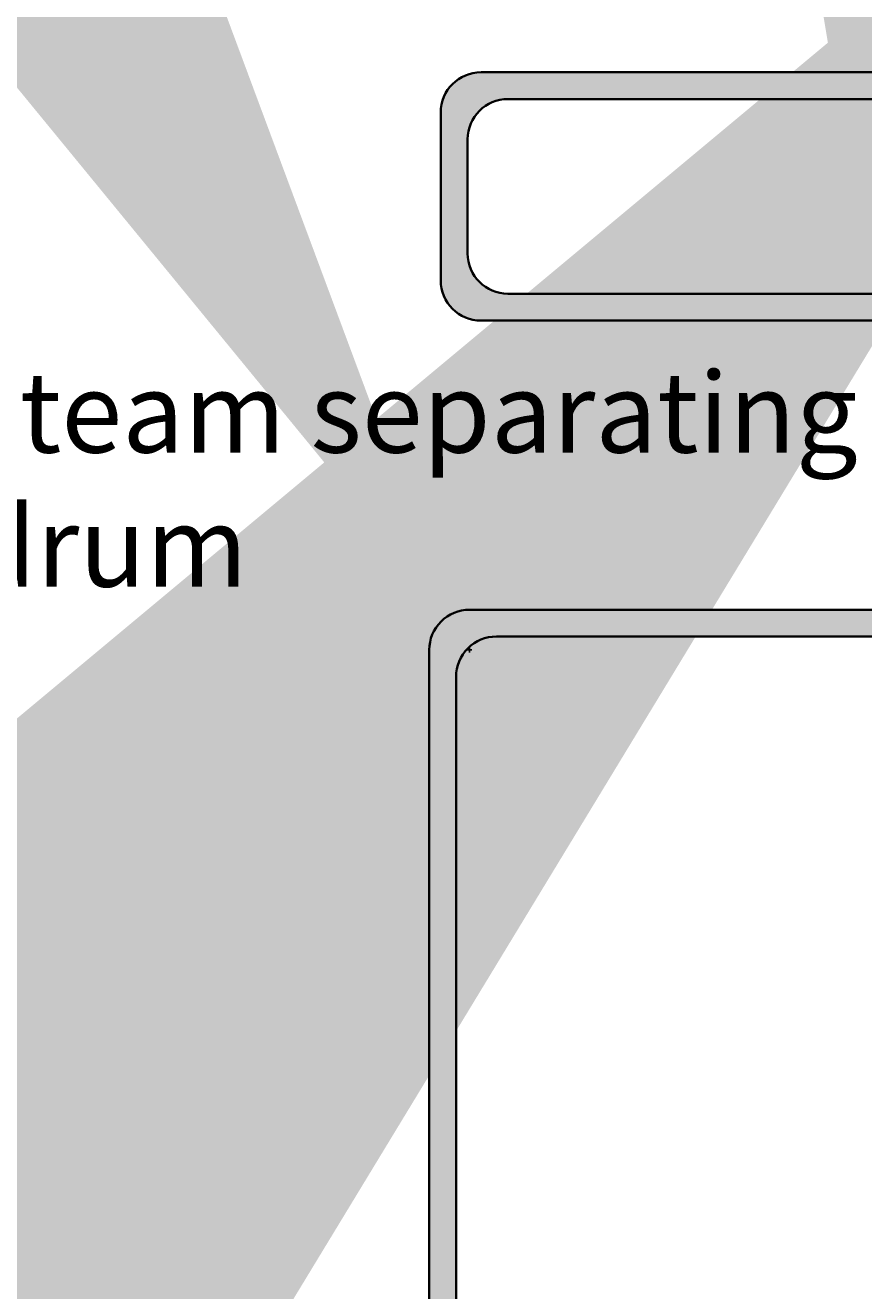
# Model space of a CAD drawing. Units: millimetres. Extents: x -22994 to 29398, y -19990 to 20176.
# Tile 16 of 135: x 5 to 37, y 52 to 99. Entities that reach past the tile are written whole.
import ezdxf

# ---------------------------------------------------------------- set-up
doc = ezdxf.new("R2010")
doc.units = ezdxf.units.MM
doc.header["$MEASUREMENT"] = 0
for name, color, linetype, lineweight in [('M-ANNO-TEXT', 7, 'Continuous', 25), ('M-DIMS', 2, 'Continuous', 18), ('M-EQPM-PATT', 7, 'Continuous', 18), ('M-PIPE', 7, 'Continuous', 35)]:
    doc.layers.add(name, color=color, linetype=linetype, lineweight=lineweight)
doc.styles.get("Standard").update_dxf_attribs({"font": 'arial.ttf'})
doc.dimstyles.get("Standard").update_dxf_attribs({"dimtxt": 0.18, "dimasz": 10000, "dimexe": 0.18, "dimexo": 0.0625, "dimgap": 0.09, "dimtad": 0, "dimtih": 1, "dimtoh": 1, "dimdec": 0, "dimzin": 0, "dimdsep": 46, "dimtxsty": 'Standard', "dimcen": 0.09, "dimadec": 0, "dimazin": 0, "dimtfac": 1, "dimtdec": 0, "dimtofl": 0, "dimtmove": 0, "dimatfit": 3, "dimfxl": 1, "dimtolj": 1, "dimtzin": 0, "dimlwd": 30, "dimarcsym": 0})

# ---------------------------------------------------------------- blocks, each defined once
blk = doc.blocks.new('*D2')
at = {"layer": 'Defpoints', "color": 0, "transparency": 16777216}
for p in [(6.677, 10.271), (290.852, 10.271), (290.852, -5.079)]:
    blk.add_point(p, dxfattribs=at)
at = {"layer": 'M-DIMS', "color": 0, "lineweight": -2, "transparency": 16777216}
for p, q in [((6.677, 10.209), (6.677, -5.259)), ((290.852, 10.209), (290.852, -5.259))]:
    blk.add_line(p, q, dxfattribs=at)
at = {"layer": 'M-DIMS', "color": 0, "lineweight": 30, "transparency": 16777216}
for p, q in [((-9993.323, -5.079), (-19993.323, -5.079)), ((10290.852, -5.079), (20290.852, -5.079))]:
    blk.add_line(p, q, dxfattribs=at)
at = {"layer": 'M-DIMS', "color": 0, "transparency": 16777216}
for points in [[(-9993.323, 1661.588), (-9993.323, -1671.745), (6.677, -5.079)], [(10290.852, 1661.588), (10290.852, -1671.745), (290.852, -5.079)]]:
    blk.add_solid(points, dxfattribs=at)
at = {"layer": 'M-DIMS', "color": 0, "transparency": 16777216, "insert": (148.765, -5.079), "char_height": 0.18, "attachment_point": 5}
blk.add_mtext('\\A1;284.2', dxfattribs=at)
blk = doc.blocks.new('*D3')
at = {"layer": 'Defpoints', "color": 0, "transparency": 16777216}
for p in [(110.265, 204.165), (110.265, 176.366), (95.833, 127.967)]:
    blk.add_point(p, dxfattribs=at)
at = {"layer": 'M-DIMS', "color": 0, "lineweight": -2, "transparency": 16777216}
for p, q in [((95.833, 128.03), (95.833, 204.345)), ((110.265, 176.429), (110.265, 204.345))]:
    blk.add_line(p, q, dxfattribs=at)
at = {"layer": 'M-DIMS', "color": 0, "lineweight": 30, "transparency": 16777216}
for p, q in [((-9904.167, 204.165), (-19904.167, 204.165)), ((10110.265, 204.165), (20110.265, 204.165))]:
    blk.add_line(p, q, dxfattribs=at)
at = {"layer": 'M-DIMS', "color": 0, "transparency": 16777216}
for points in [[(-9904.167, 1870.832), (-9904.167, -1462.501), (95.833, 204.165)], [(10110.265, 1870.832), (10110.265, -1462.501), (110.265, 204.165)]]:
    blk.add_solid(points, dxfattribs=at)
at = {"layer": 'M-DIMS', "color": 0, "transparency": 16777216, "insert": (103.049, 204.165), "char_height": 0.18, "attachment_point": 5}
blk.add_mtext('\\A1;14.432', dxfattribs=at)
blk = doc.blocks.new('*D4')
at = {"layer": 'Defpoints', "color": 0, "transparency": 16777216}
for p in [(116.265, 204.165), (110.265, 176.366), (116.265, 176.366)]:
    blk.add_point(p, dxfattribs=at)
at = {"layer": 'M-DIMS', "color": 0, "lineweight": -2, "transparency": 16777216}
for p, q in [((110.265, 176.429), (110.265, 204.345)), ((116.265, 176.429), (116.265, 204.345))]:
    blk.add_line(p, q, dxfattribs=at)
at = {"layer": 'M-DIMS', "color": 0, "lineweight": 30, "transparency": 16777216}
for p, q in [((-9889.735, 204.165), (-19889.735, 204.165)), ((10116.265, 204.165), (20116.265, 204.165))]:
    blk.add_line(p, q, dxfattribs=at)
at = {"layer": 'M-DIMS', "color": 0, "transparency": 16777216}
for points in [[(-9889.735, 1870.832), (-9889.735, -1462.501), (110.265, 204.165)], [(10116.265, 1870.832), (10116.265, -1462.501), (116.265, 204.165)]]:
    blk.add_solid(points, dxfattribs=at)
at = {"layer": 'M-DIMS', "color": 0, "transparency": 16777216, "insert": (113.265, 204.165), "char_height": 0.18, "attachment_point": 5}
blk.add_mtext('\\A1;6', dxfattribs=at)
blk = doc.blocks.new('*D5')
at = {"layer": 'Defpoints', "color": 0, "transparency": 16777216}
for p in [(181.265, 204.165), (116.265, 176.366), (181.265, 176.366)]:
    blk.add_point(p, dxfattribs=at)
at = {"layer": 'M-DIMS', "color": 0, "lineweight": -2, "transparency": 16777216}
for p, q in [((116.265, 176.429), (116.265, 204.345)), ((181.265, 176.429), (181.265, 204.345))]:
    blk.add_line(p, q, dxfattribs=at)
at = {"layer": 'M-DIMS', "color": 0, "lineweight": 30, "transparency": 16777216}
for p, q in [((-9883.735, 204.165), (-19883.735, 204.165)), ((10181.265, 204.165), (20181.265, 204.165))]:
    blk.add_line(p, q, dxfattribs=at)
at = {"layer": 'M-DIMS', "color": 0, "transparency": 16777216}
for points in [[(-9883.735, 1870.832), (-9883.735, -1462.501), (116.265, 204.165)], [(10181.265, 1870.832), (10181.265, -1462.501), (181.265, 204.165)]]:
    blk.add_solid(points, dxfattribs=at)
at = {"layer": 'M-DIMS', "color": 0, "transparency": 16777216, "insert": (148.765, 204.165), "char_height": 0.18, "attachment_point": 5}
blk.add_mtext('\\A1;65', dxfattribs=at)
blk = doc.blocks.new('*D6')
at = {"layer": 'Defpoints', "color": 0, "transparency": 16777216}
for p in [(187.265, 204.165), (181.265, 176.366), (187.265, 176.366)]:
    blk.add_point(p, dxfattribs=at)
at = {"layer": 'M-DIMS', "color": 0, "lineweight": -2, "transparency": 16777216}
for p, q in [((181.265, 176.429), (181.265, 204.345)), ((187.265, 176.429), (187.265, 204.345))]:
    blk.add_line(p, q, dxfattribs=at)
at = {"layer": 'M-DIMS', "color": 0, "lineweight": 30, "transparency": 16777216}
for p, q in [((-9818.735, 204.165), (-19818.735, 204.165)), ((10187.265, 204.165), (20187.265, 204.165))]:
    blk.add_line(p, q, dxfattribs=at)
at = {"layer": 'M-DIMS', "color": 0, "transparency": 16777216}
for points in [[(-9818.735, 1870.832), (-9818.735, -1462.501), (181.265, 204.165)], [(10187.265, 1870.832), (10187.265, -1462.501), (187.265, 204.165)]]:
    blk.add_solid(points, dxfattribs=at)
at = {"layer": 'M-DIMS', "color": 0, "transparency": 16777216, "insert": (184.265, 204.165), "char_height": 0.18, "attachment_point": 5}
blk.add_mtext('\\A1;6', dxfattribs=at)
blk = doc.blocks.new('*D7')
at = {"layer": 'Defpoints', "color": 0, "transparency": 16777216}
for p in [(201.697, 204.165), (187.265, 176.366), (201.697, 127.967)]:
    blk.add_point(p, dxfattribs=at)
at = {"layer": 'M-DIMS', "color": 0, "lineweight": -2, "transparency": 16777216}
for p, q in [((187.265, 176.429), (187.265, 204.345)), ((201.697, 128.03), (201.697, 204.345))]:
    blk.add_line(p, q, dxfattribs=at)
at = {"layer": 'M-DIMS', "color": 0, "lineweight": 30, "transparency": 16777216}
for p, q in [((-9812.735, 204.165), (-19812.735, 204.165)), ((10201.697, 204.165), (20201.697, 204.165))]:
    blk.add_line(p, q, dxfattribs=at)
at = {"layer": 'M-DIMS', "color": 0, "transparency": 16777216}
for points in [[(-9812.735, 1870.832), (-9812.735, -1462.501), (187.265, 204.165)], [(10201.697, 1870.832), (10201.697, -1462.501), (201.697, 204.165)]]:
    blk.add_solid(points, dxfattribs=at)
at = {"layer": 'M-DIMS', "color": 0, "transparency": 16777216, "insert": (194.481, 204.165), "char_height": 0.18, "attachment_point": 5}
blk.add_mtext('\\A1;14.432', dxfattribs=at)
blk = doc.blocks.new('*D8')
at = {"layer": 'Defpoints', "color": 0, "transparency": 16777216}
for p in [(227.648, 204.165), (227.648, 146.73), (201.697, 127.967)]:
    blk.add_point(p, dxfattribs=at)
at = {"layer": 'M-DIMS', "color": 0, "lineweight": -2, "transparency": 16777216}
for p, q in [((201.697, 128.03), (201.697, 204.345)), ((227.648, 146.792), (227.648, 204.345))]:
    blk.add_line(p, q, dxfattribs=at)
at = {"layer": 'M-DIMS', "color": 0, "lineweight": 30, "transparency": 16777216}
for p, q in [((-9798.303, 204.165), (-19798.303, 204.165)), ((10227.648, 204.165), (20227.648, 204.165))]:
    blk.add_line(p, q, dxfattribs=at)
at = {"layer": 'M-DIMS', "color": 0, "transparency": 16777216}
for points in [[(-9798.303, 1870.832), (-9798.303, -1462.501), (201.697, 204.165)], [(10227.648, 1870.832), (10227.648, -1462.501), (227.648, 204.165)]]:
    blk.add_solid(points, dxfattribs=at)
at = {"layer": 'M-DIMS', "color": 0, "transparency": 16777216, "insert": (214.673, 204.165), "char_height": 0.18, "attachment_point": 5}
blk.add_mtext('\\A1;25.95', dxfattribs=at)
blk = doc.blocks.new('*D9')
at = {"layer": 'Defpoints', "color": 0, "transparency": 16777216}
for p in [(187.265, 176.366), (306.202, 176.366), (290.852, 10.271)]:
    blk.add_point(p, dxfattribs=at)
at = {"layer": 'M-DIMS', "color": 0, "lineweight": 30, "transparency": 16777216}
for p, q in [((306.202, 10176.366), (306.202, 20176.366)), ((306.202, -9989.729), (306.202, -19989.729))]:
    blk.add_line(p, q, dxfattribs=at)
at = {"layer": 'M-DIMS', "color": 0, "lineweight": -2, "transparency": 16777216}
for p, q in [((187.327, 176.366), (306.382, 176.366)), ((290.915, 10.271), (306.382, 10.271))]:
    blk.add_line(p, q, dxfattribs=at)
at = {"layer": 'M-DIMS', "color": 0, "transparency": 16777216}
for points in [[(-1360.465, 10176.366), (1972.869, 10176.366), (306.202, 176.366)], [(-1360.465, -9989.729), (1972.869, -9989.729), (306.202, 10.271)]]:
    blk.add_solid(points, dxfattribs=at)
at = {"layer": 'M-DIMS', "color": 0, "transparency": 16777216, "insert": (306.202, 93.319), "char_height": 0.18, "attachment_point": 5}
blk.add_mtext('\\A1;166.1', dxfattribs=at)
blk = doc.blocks.new('*D10')
at = {"layer": 'Defpoints', "color": 0, "transparency": 16777216}
for p in [(125.65, 136.071), (133.346, 136.071), (133.346, -5.079)]:
    blk.add_point(p, dxfattribs=at)
at = {"layer": 'M-DIMS', "color": 0, "lineweight": -2, "transparency": 16777216}
for p, q in [((125.65, 136.009), (125.65, -5.259)), ((133.346, 136.009), (133.346, -5.259))]:
    blk.add_line(p, q, dxfattribs=at)
at = {"layer": 'M-DIMS', "color": 0, "lineweight": 30, "transparency": 16777216}
for p, q in [((-9874.35, -5.079), (-19874.35, -5.079)), ((10133.346, -5.079), (20133.346, -5.079))]:
    blk.add_line(p, q, dxfattribs=at)
at = {"layer": 'M-DIMS', "color": 0, "transparency": 16777216}
for points in [[(-9874.35, 1661.588), (-9874.35, -1671.745), (125.65, -5.079)], [(10133.346, 1661.588), (10133.346, -1671.745), (133.346, -5.079)]]:
    blk.add_solid(points, dxfattribs=at)
at = {"layer": 'M-DIMS', "color": 0, "transparency": 16777216, "insert": (129.498, -5.079), "char_height": 0.18, "attachment_point": 5}
blk.add_mtext('\\A1;7.696', dxfattribs=at)
blk = doc.blocks.new('*D11')
at = {"layer": 'Defpoints', "color": 0, "transparency": 16777216}
for p in [(133.346, 136.071), (135.65, 136.071), (135.65, -5.079)]:
    blk.add_point(p, dxfattribs=at)
at = {"layer": 'M-DIMS', "color": 0, "lineweight": -2, "transparency": 16777216}
for p, q in [((133.346, 136.009), (133.346, -5.259)), ((135.65, 136.009), (135.65, -5.259))]:
    blk.add_line(p, q, dxfattribs=at)
at = {"layer": 'M-DIMS', "color": 0, "lineweight": 30, "transparency": 16777216}
for p, q in [((-9866.654, -5.079), (-19866.654, -5.079)), ((10135.65, -5.079), (20135.65, -5.079))]:
    blk.add_line(p, q, dxfattribs=at)
at = {"layer": 'M-DIMS', "color": 0, "transparency": 16777216}
for points in [[(-9866.654, 1661.588), (-9866.654, -1671.745), (133.346, -5.079)], [(10135.65, 1661.588), (10135.65, -1671.745), (135.65, -5.079)]]:
    blk.add_solid(points, dxfattribs=at)
at = {"layer": 'M-DIMS', "color": 0, "transparency": 16777216, "insert": (134.498, -5.079), "char_height": 0.18, "attachment_point": 5}
blk.add_mtext('\\A1;2.304', dxfattribs=at)
blk = doc.blocks.new('*D12')
at = {"layer": 'Defpoints', "color": 0, "transparency": 16777216}
for p in [(135.65, 136.071), (145.65, 136.071), (145.65, -5.079)]:
    blk.add_point(p, dxfattribs=at)
at = {"layer": 'M-DIMS', "color": 0, "lineweight": -2, "transparency": 16777216}
for p, q in [((135.65, 136.009), (135.65, -5.259)), ((145.65, 136.009), (145.65, -5.259))]:
    blk.add_line(p, q, dxfattribs=at)
at = {"layer": 'M-DIMS', "color": 0, "lineweight": 30, "transparency": 16777216}
for p, q in [((-9864.35, -5.079), (-19864.35, -5.079)), ((10145.65, -5.079), (20145.65, -5.079))]:
    blk.add_line(p, q, dxfattribs=at)
at = {"layer": 'M-DIMS', "color": 0, "transparency": 16777216}
for points in [[(-9864.35, 1661.588), (-9864.35, -1671.745), (135.65, -5.079)], [(10145.65, 1661.588), (10145.65, -1671.745), (145.65, -5.079)]]:
    blk.add_solid(points, dxfattribs=at)
at = {"layer": 'M-DIMS', "color": 0, "transparency": 16777216, "insert": (140.65, -5.079), "char_height": 0.18, "attachment_point": 5}
blk.add_mtext('\\A1;10', dxfattribs=at)
blk = doc.blocks.new('*D13')
at = {"layer": 'Defpoints', "color": 0, "transparency": 16777216}
for p in [(145.65, 136.071), (155.65, 136.071), (155.65, -5.079)]:
    blk.add_point(p, dxfattribs=at)
at = {"layer": 'M-DIMS', "color": 0, "lineweight": -2, "transparency": 16777216}
for p, q in [((145.65, 136.009), (145.65, -5.259)), ((155.65, 136.009), (155.65, -5.259))]:
    blk.add_line(p, q, dxfattribs=at)
at = {"layer": 'M-DIMS', "color": 0, "lineweight": 30, "transparency": 16777216}
for p, q in [((-9854.35, -5.079), (-19854.35, -5.079)), ((10155.65, -5.079), (20155.65, -5.079))]:
    blk.add_line(p, q, dxfattribs=at)
at = {"layer": 'M-DIMS', "color": 0, "transparency": 16777216}
for points in [[(-9854.35, 1661.588), (-9854.35, -1671.745), (145.65, -5.079)], [(10155.65, 1661.588), (10155.65, -1671.745), (155.65, -5.079)]]:
    blk.add_solid(points, dxfattribs=at)
at = {"layer": 'M-DIMS', "color": 0, "transparency": 16777216, "insert": (150.65, -5.079), "char_height": 0.18, "attachment_point": 5}
blk.add_mtext('\\A1;10', dxfattribs=at)
blk = doc.blocks.new('*D14')
at = {"layer": 'Defpoints', "color": 0, "transparency": 16777216}
for p in [(155.65, 136.071), (165.65, 136.071), (165.65, -5.079)]:
    blk.add_point(p, dxfattribs=at)
at = {"layer": 'M-DIMS', "color": 0, "lineweight": -2, "transparency": 16777216}
for p, q in [((155.65, 136.009), (155.65, -5.259)), ((165.65, 136.009), (165.65, -5.259))]:
    blk.add_line(p, q, dxfattribs=at)
at = {"layer": 'M-DIMS', "color": 0, "lineweight": 30, "transparency": 16777216}
for p, q in [((-9844.35, -5.079), (-19844.35, -5.079)), ((10165.65, -5.079), (20165.65, -5.079))]:
    blk.add_line(p, q, dxfattribs=at)
at = {"layer": 'M-DIMS', "color": 0, "transparency": 16777216}
for points in [[(-9844.35, 1661.588), (-9844.35, -1671.745), (155.65, -5.079)], [(10165.65, 1661.588), (10165.65, -1671.745), (165.65, -5.079)]]:
    blk.add_solid(points, dxfattribs=at)
at = {"layer": 'M-DIMS', "color": 0, "transparency": 16777216, "insert": (160.65, -5.079), "char_height": 0.18, "attachment_point": 5}
blk.add_mtext('\\A1;10', dxfattribs=at)
blk = doc.blocks.new('*D15')
at = {"layer": 'Defpoints', "color": 0, "transparency": 16777216}
for p in [(173.346, 154.788), (173.346, 136.071), (306.202, 136.071)]:
    blk.add_point(p, dxfattribs=at)
at = {"layer": 'M-DIMS', "color": 0, "lineweight": 30, "transparency": 16777216}
for p, q in [((306.202, 10154.788), (306.202, 20154.788)), ((306.202, -9863.929), (306.202, -19863.929))]:
    blk.add_line(p, q, dxfattribs=at)
at = {"layer": 'M-DIMS', "color": 0, "lineweight": -2, "transparency": 16777216}
for p, q in [((173.408, 154.788), (306.382, 154.788)), ((173.408, 136.071), (306.382, 136.071))]:
    blk.add_line(p, q, dxfattribs=at)
at = {"layer": 'M-DIMS', "color": 0, "transparency": 16777216}
for points in [[(-1360.465, 10154.788), (1972.869, 10154.788), (306.202, 154.788)], [(-1360.465, -9863.929), (1972.869, -9863.929), (306.202, 136.071)]]:
    blk.add_solid(points, dxfattribs=at)
at = {"layer": 'M-DIMS', "color": 0, "transparency": 16777216, "insert": (306.202, 145.43), "char_height": 0.18, "attachment_point": 5}
blk.add_mtext('\\A1;18.717', dxfattribs=at)
blk = doc.blocks.new('*D16')
at = {"layer": 'Defpoints', "color": 0, "transparency": 16777216}
for p in [(120.17, 204.165), (110.466, 48.035), (120.17, 48.035)]:
    blk.add_point(p, dxfattribs=at)
at = {"layer": 'M-DIMS', "color": 0, "lineweight": -2, "transparency": 16777216}
for p, q in [((110.466, 48.097), (110.466, 204.345)), ((120.17, 48.097), (120.17, 204.345))]:
    blk.add_line(p, q, dxfattribs=at)
at = {"layer": 'M-DIMS', "color": 0, "lineweight": 30, "transparency": 16777216}
for p, q in [((-9889.534, 204.165), (-19889.534, 204.165)), ((10120.17, 204.165), (20120.17, 204.165))]:
    blk.add_line(p, q, dxfattribs=at)
at = {"layer": 'M-DIMS', "color": 0, "transparency": 16777216}
for points in [[(-9889.534, 1870.832), (-9889.534, -1462.501), (110.466, 204.165)], [(10120.17, 1870.832), (10120.17, -1462.501), (120.17, 204.165)]]:
    blk.add_solid(points, dxfattribs=at)
at = {"layer": 'M-DIMS', "color": 0, "transparency": 16777216, "insert": (115.318, 204.165), "char_height": 0.18, "attachment_point": 5}
blk.add_mtext('\\A1;9.704', dxfattribs=at)
blk = doc.blocks.new('*D17')
at = {"layer": 'Defpoints', "color": 0, "transparency": 16777216}
for p in [(126.17, 204.165), (120.17, 48.035), (126.17, 48.035)]:
    blk.add_point(p, dxfattribs=at)
at = {"layer": 'M-DIMS', "color": 0, "lineweight": -2, "transparency": 16777216}
for p, q in [((120.17, 48.097), (120.17, 204.345)), ((126.17, 48.097), (126.17, 204.345))]:
    blk.add_line(p, q, dxfattribs=at)
at = {"layer": 'M-DIMS', "color": 0, "lineweight": 30, "transparency": 16777216}
for p, q in [((-9879.83, 204.165), (-19879.83, 204.165)), ((10126.17, 204.165), (20126.17, 204.165))]:
    blk.add_line(p, q, dxfattribs=at)
at = {"layer": 'M-DIMS', "color": 0, "transparency": 16777216}
for points in [[(-9879.83, 1870.832), (-9879.83, -1462.501), (120.17, 204.165)], [(10126.17, 1870.832), (10126.17, -1462.501), (126.17, 204.165)]]:
    blk.add_solid(points, dxfattribs=at)
at = {"layer": 'M-DIMS', "color": 0, "transparency": 16777216, "insert": (123.17, 204.165), "char_height": 0.18, "attachment_point": 5}
blk.add_mtext('\\A1;6', dxfattribs=at)
blk = doc.blocks.new('*D18')
at = {"layer": 'Defpoints', "color": 0, "transparency": 16777216}
for p in [(132.17, 204.165), (126.17, 48.035), (132.17, 48.035)]:
    blk.add_point(p, dxfattribs=at)
at = {"layer": 'M-DIMS', "color": 0, "lineweight": -2, "transparency": 16777216}
for p, q in [((126.17, 48.097), (126.17, 204.345)), ((132.17, 48.097), (132.17, 204.345))]:
    blk.add_line(p, q, dxfattribs=at)
at = {"layer": 'M-DIMS', "color": 0, "lineweight": 30, "transparency": 16777216}
for p, q in [((-9873.83, 204.165), (-19873.83, 204.165)), ((10132.17, 204.165), (20132.17, 204.165))]:
    blk.add_line(p, q, dxfattribs=at)
at = {"layer": 'M-DIMS', "color": 0, "transparency": 16777216}
for points in [[(-9873.83, 1870.832), (-9873.83, -1462.501), (126.17, 204.165)], [(10132.17, 1870.832), (10132.17, -1462.501), (132.17, 204.165)]]:
    blk.add_solid(points, dxfattribs=at)
at = {"layer": 'M-DIMS', "color": 0, "transparency": 16777216, "insert": (129.17, 204.165), "char_height": 0.18, "attachment_point": 5}
blk.add_mtext('\\A1;6', dxfattribs=at)
blk = doc.blocks.new('*D19')
at = {"layer": 'Defpoints', "color": 0, "transparency": 16777216}
for p in [(138.17, 204.165), (132.17, 48.035), (138.17, 48.035)]:
    blk.add_point(p, dxfattribs=at)
at = {"layer": 'M-DIMS', "color": 0, "lineweight": -2, "transparency": 16777216}
for p, q in [((132.17, 48.097), (132.17, 204.345)), ((138.17, 48.097), (138.17, 204.345))]:
    blk.add_line(p, q, dxfattribs=at)
at = {"layer": 'M-DIMS', "color": 0, "lineweight": 30, "transparency": 16777216}
for p, q in [((-9867.83, 204.165), (-19867.83, 204.165)), ((10138.17, 204.165), (20138.17, 204.165))]:
    blk.add_line(p, q, dxfattribs=at)
at = {"layer": 'M-DIMS', "color": 0, "transparency": 16777216}
for points in [[(-9867.83, 1870.832), (-9867.83, -1462.501), (132.17, 204.165)], [(10138.17, 1870.832), (10138.17, -1462.501), (138.17, 204.165)]]:
    blk.add_solid(points, dxfattribs=at)
at = {"layer": 'M-DIMS', "color": 0, "transparency": 16777216, "insert": (135.17, 204.165), "char_height": 0.18, "attachment_point": 5}
blk.add_mtext('\\A1;6', dxfattribs=at)
blk = doc.blocks.new('*D20')
at = {"layer": 'Defpoints', "color": 0, "transparency": 16777216}
for p in [(144.17, 204.165), (138.17, 48.035), (144.17, 48.035)]:
    blk.add_point(p, dxfattribs=at)
at = {"layer": 'M-DIMS', "color": 0, "lineweight": -2, "transparency": 16777216}
for p, q in [((138.17, 48.097), (138.17, 204.345)), ((144.17, 48.097), (144.17, 204.345))]:
    blk.add_line(p, q, dxfattribs=at)
at = {"layer": 'M-DIMS', "color": 0, "lineweight": 30, "transparency": 16777216}
for p, q in [((-9861.83, 204.165), (-19861.83, 204.165)), ((10144.17, 204.165), (20144.17, 204.165))]:
    blk.add_line(p, q, dxfattribs=at)
at = {"layer": 'M-DIMS', "color": 0, "transparency": 16777216}
for points in [[(-9861.83, 1870.832), (-9861.83, -1462.501), (138.17, 204.165)], [(10144.17, 1870.832), (10144.17, -1462.501), (144.17, 204.165)]]:
    blk.add_solid(points, dxfattribs=at)
at = {"layer": 'M-DIMS', "color": 0, "transparency": 16777216, "insert": (141.17, 204.165), "char_height": 0.18, "attachment_point": 5}
blk.add_mtext('\\A1;6', dxfattribs=at)
blk = doc.blocks.new('*D21')
at = {"layer": 'Defpoints', "color": 0, "transparency": 16777216}
for p in [(149.116, 204.165), (144.17, 48.035), (149.116, 48.035)]:
    blk.add_point(p, dxfattribs=at)
at = {"layer": 'M-DIMS', "color": 0, "lineweight": -2, "transparency": 16777216}
for p, q in [((144.17, 48.097), (144.17, 204.345)), ((149.116, 48.097), (149.116, 204.345))]:
    blk.add_line(p, q, dxfattribs=at)
at = {"layer": 'M-DIMS', "color": 0, "lineweight": 30, "transparency": 16777216}
for p, q in [((-9855.83, 204.165), (-19855.83, 204.165)), ((10149.116, 204.165), (20149.116, 204.165))]:
    blk.add_line(p, q, dxfattribs=at)
at = {"layer": 'M-DIMS', "color": 0, "transparency": 16777216}
for points in [[(-9855.83, 1870.832), (-9855.83, -1462.501), (144.17, 204.165)], [(10149.116, 1870.832), (10149.116, -1462.501), (149.116, 204.165)]]:
    blk.add_solid(points, dxfattribs=at)
at = {"layer": 'M-DIMS', "color": 0, "transparency": 16777216, "insert": (146.643, 204.165), "char_height": 0.18, "attachment_point": 5}
blk.add_mtext('\\A1;4.945', dxfattribs=at)
blk = doc.blocks.new('*D22')
at = {"layer": 'Defpoints', "color": 0, "transparency": 16777216}
for p in [(149.116, 30.99), (155.116, 30.99), (155.116, -5.079)]:
    blk.add_point(p, dxfattribs=at)
at = {"layer": 'M-DIMS', "color": 0, "lineweight": -2, "transparency": 16777216}
for p, q in [((149.116, 30.927), (149.116, -5.259)), ((155.116, 30.927), (155.116, -5.259))]:
    blk.add_line(p, q, dxfattribs=at)
at = {"layer": 'M-DIMS', "color": 0, "lineweight": 30, "transparency": 16777216}
for p, q in [((-9850.884, -5.079), (-19850.884, -5.079)), ((10155.116, -5.079), (20155.116, -5.079))]:
    blk.add_line(p, q, dxfattribs=at)
at = {"layer": 'M-DIMS', "color": 0, "transparency": 16777216}
for points in [[(-9850.884, 1661.588), (-9850.884, -1671.745), (149.116, -5.079)], [(10155.116, 1661.588), (10155.116, -1671.745), (155.116, -5.079)]]:
    blk.add_solid(points, dxfattribs=at)
at = {"layer": 'M-DIMS', "color": 0, "transparency": 16777216, "insert": (152.116, -5.079), "char_height": 0.18, "attachment_point": 5}
blk.add_mtext('\\A1;6', dxfattribs=at)
blk = doc.blocks.new('*D23')
at = {"layer": 'Defpoints', "color": 0, "transparency": 16777216}
for p in [(155.116, 30.99), (161.116, 30.99), (161.116, -5.079)]:
    blk.add_point(p, dxfattribs=at)
at = {"layer": 'M-DIMS', "color": 0, "lineweight": -2, "transparency": 16777216}
for p, q in [((155.116, 30.927), (155.116, -5.259)), ((161.116, 30.927), (161.116, -5.259))]:
    blk.add_line(p, q, dxfattribs=at)
at = {"layer": 'M-DIMS', "color": 0, "lineweight": 30, "transparency": 16777216}
for p, q in [((-9844.884, -5.079), (-19844.884, -5.079)), ((10161.116, -5.079), (20161.116, -5.079))]:
    blk.add_line(p, q, dxfattribs=at)
at = {"layer": 'M-DIMS', "color": 0, "transparency": 16777216}
for points in [[(-9844.884, 1661.588), (-9844.884, -1671.745), (155.116, -5.079)], [(10161.116, 1661.588), (10161.116, -1671.745), (161.116, -5.079)]]:
    blk.add_solid(points, dxfattribs=at)
at = {"layer": 'M-DIMS', "color": 0, "transparency": 16777216, "insert": (158.116, -5.079), "char_height": 0.18, "attachment_point": 5}
blk.add_mtext('\\A1;6', dxfattribs=at)
blk = doc.blocks.new('*D24')
at = {"layer": 'Defpoints', "color": 0, "transparency": 16777216}
for p in [(161.116, 30.99), (166.439, 30.99), (166.439, -5.079)]:
    blk.add_point(p, dxfattribs=at)
at = {"layer": 'M-DIMS', "color": 0, "lineweight": -2, "transparency": 16777216}
for p, q in [((161.116, 30.927), (161.116, -5.259)), ((166.439, 30.927), (166.439, -5.259))]:
    blk.add_line(p, q, dxfattribs=at)
at = {"layer": 'M-DIMS', "color": 0, "lineweight": 30, "transparency": 16777216}
for p, q in [((-9838.884, -5.079), (-19838.884, -5.079)), ((10166.439, -5.079), (20166.439, -5.079))]:
    blk.add_line(p, q, dxfattribs=at)
at = {"layer": 'M-DIMS', "color": 0, "transparency": 16777216}
for points in [[(-9838.884, 1661.588), (-9838.884, -1671.745), (161.116, -5.079)], [(10166.439, 1661.588), (10166.439, -1671.745), (166.439, -5.079)]]:
    blk.add_solid(points, dxfattribs=at)
at = {"layer": 'M-DIMS', "color": 0, "transparency": 16777216, "insert": (163.777, -5.079), "char_height": 0.18, "attachment_point": 5}
blk.add_mtext('\\A1;5.323', dxfattribs=at)
blk = doc.blocks.new('*D25')
at = {"layer": 'Defpoints', "color": 0, "transparency": 16777216}
for p in [(166.439, 30.99), (172.439, 30.99), (172.439, -5.079)]:
    blk.add_point(p, dxfattribs=at)
at = {"layer": 'M-DIMS', "color": 0, "lineweight": -2, "transparency": 16777216}
for p, q in [((166.439, 30.927), (166.439, -5.259)), ((172.439, 30.927), (172.439, -5.259))]:
    blk.add_line(p, q, dxfattribs=at)
at = {"layer": 'M-DIMS', "color": 0, "lineweight": 30, "transparency": 16777216}
for p, q in [((-9833.561, -5.079), (-19833.561, -5.079)), ((10172.439, -5.079), (20172.439, -5.079))]:
    blk.add_line(p, q, dxfattribs=at)
at = {"layer": 'M-DIMS', "color": 0, "transparency": 16777216}
for points in [[(-9833.561, 1661.588), (-9833.561, -1671.745), (166.439, -5.079)], [(10172.439, 1661.588), (10172.439, -1671.745), (172.439, -5.079)]]:
    blk.add_solid(points, dxfattribs=at)
at = {"layer": 'M-DIMS', "color": 0, "transparency": 16777216, "insert": (169.439, -5.079), "char_height": 0.18, "attachment_point": 5}
blk.add_mtext('\\A1;6', dxfattribs=at)
blk = doc.blocks.new('*D26')
at = {"layer": 'Defpoints', "color": 0, "transparency": 16777216}
for p in [(172.439, 30.99), (178.439, 30.99), (178.439, -5.079)]:
    blk.add_point(p, dxfattribs=at)
at = {"layer": 'M-DIMS', "color": 0, "lineweight": -2, "transparency": 16777216}
for p, q in [((172.439, 30.927), (172.439, -5.259)), ((178.439, 30.927), (178.439, -5.259))]:
    blk.add_line(p, q, dxfattribs=at)
at = {"layer": 'M-DIMS', "color": 0, "lineweight": 30, "transparency": 16777216}
for p, q in [((-9827.561, -5.079), (-19827.561, -5.079)), ((10178.439, -5.079), (20178.439, -5.079))]:
    blk.add_line(p, q, dxfattribs=at)
at = {"layer": 'M-DIMS', "color": 0, "transparency": 16777216}
for points in [[(-9827.561, 1661.588), (-9827.561, -1671.745), (172.439, -5.079)], [(10178.439, 1661.588), (10178.439, -1671.745), (178.439, -5.079)]]:
    blk.add_solid(points, dxfattribs=at)
at = {"layer": 'M-DIMS', "color": 0, "transparency": 16777216, "insert": (175.439, -5.079), "char_height": 0.18, "attachment_point": 5}
blk.add_mtext('\\A1;6', dxfattribs=at)
blk = doc.blocks.new('*D27')
at = {"layer": 'Defpoints', "color": 0, "transparency": 16777216}
for p in [(178.439, 30.99), (188.117, 30.99), (188.117, -5.079)]:
    blk.add_point(p, dxfattribs=at)
at = {"layer": 'M-DIMS', "color": 0, "lineweight": -2, "transparency": 16777216}
for p, q in [((178.439, 30.927), (178.439, -5.259)), ((188.117, 30.927), (188.117, -5.259))]:
    blk.add_line(p, q, dxfattribs=at)
at = {"layer": 'M-DIMS', "color": 0, "lineweight": 30, "transparency": 16777216}
for p, q in [((-9821.561, -5.079), (-19821.561, -5.079)), ((10188.117, -5.079), (20188.117, -5.079))]:
    blk.add_line(p, q, dxfattribs=at)
at = {"layer": 'M-DIMS', "color": 0, "transparency": 16777216}
for points in [[(-9821.561, 1661.588), (-9821.561, -1671.745), (178.439, -5.079)], [(10188.117, 1661.588), (10188.117, -1671.745), (188.117, -5.079)]]:
    blk.add_solid(points, dxfattribs=at)
at = {"layer": 'M-DIMS', "color": 0, "transparency": 16777216, "insert": (183.278, -5.079), "char_height": 0.18, "attachment_point": 5}
blk.add_mtext('\\A1;9.679', dxfattribs=at)
blk = doc.blocks.new('*D28')
at = {"layer": 'Defpoints', "color": 0, "transparency": 16777216}
for p in [(188.117, 48.035), (306.202, 48.035), (188.117, 30.99)]:
    blk.add_point(p, dxfattribs=at)
at = {"layer": 'M-DIMS', "color": 0, "lineweight": 30, "transparency": 16777216}
for p, q in [((306.202, 10048.035), (306.202, 20048.035)), ((306.202, -9969.01), (306.202, -19969.01))]:
    blk.add_line(p, q, dxfattribs=at)
at = {"layer": 'M-DIMS', "color": 0, "lineweight": -2, "transparency": 16777216}
for p, q in [((188.18, 48.035), (306.382, 48.035)), ((188.18, 30.99), (306.382, 30.99))]:
    blk.add_line(p, q, dxfattribs=at)
at = {"layer": 'M-DIMS', "color": 0, "transparency": 16777216}
for points in [[(-1360.465, 10048.035), (1972.869, 10048.035), (306.202, 48.035)], [(-1360.465, -9969.01), (1972.869, -9969.01), (306.202, 30.99)]]:
    blk.add_solid(points, dxfattribs=at)
at = {"layer": 'M-DIMS', "color": 0, "transparency": 16777216, "insert": (306.202, 39.512), "char_height": 0.18, "attachment_point": 5}
blk.add_mtext('\\A1;17.045', dxfattribs=at)
blk = doc.blocks.new('*D32')
at = {"layer": 'Defpoints', "color": 0, "transparency": 16777216}
for p in [(57.164, 118.614), (52.413, 113.093)]:
    blk.add_point(p, dxfattribs=at)
at = {"layer": 'M-DIMS', "color": 0, "lineweight": -2, "transparency": 16777216}
for p, q in [((57.074, 118.614), (57.254, 118.614)), ((57.164, 118.524), (57.164, 118.704))]:
    blk.add_line(p, q, dxfattribs=at)
at = {"layer": 'M-DIMS', "color": 0, "lineweight": 30, "transparency": 16777216}
for p, q in [((-12992.534, -15047.031), (-6470.06, -7466.969)), ((-22992.534, -15047.031), (-12992.534, -15047.031))]:
    blk.add_line(p, q, dxfattribs=at)
at = {"layer": 'M-DIMS', "color": 0, "transparency": 16777216}
blk.add_solid([(-7733.404, -6379.89), (-5206.717, -8554.048), (52.413, 113.093)], dxfattribs=at)
at = {"layer": 'M-DIMS', "color": 0, "transparency": 16777216, "insert": (-22993.208, -15047.031), "char_height": 0.18, "attachment_point": 5}
blk.add_mtext('\\A1;2X R7.284', dxfattribs=at)
blk = doc.blocks.new('*D35')
at = {"layer": 'Defpoints', "color": 0, "transparency": 16777216}
for p in [(21.093, 77.393), (21.84, 76.092)]:
    blk.add_point(p, dxfattribs=at)
at = {"layer": 'M-DIMS', "color": 0, "lineweight": 30, "transparency": 16777216}
for p, q in [((-19938.013, 17421.447), (-9938.013, 17421.447)), ((-9938.013, 17421.447), (-4958.46, 8749.42))]:
    blk.add_line(p, q, dxfattribs=at)
at = {"layer": 'M-DIMS', "color": 0, "lineweight": -2, "transparency": 16777216}
for p, q in [((21.75, 76.092), (21.93, 76.092)), ((21.84, 76.002), (21.84, 76.182))]:
    blk.add_line(p, q, dxfattribs=at)
at = {"layer": 'M-DIMS', "color": 0, "transparency": 16777216}
blk.add_solid([(-3513.122, 9579.345), (-6403.798, 7919.494), (21.093, 77.393)], dxfattribs=at)
at = {"layer": 'M-DIMS', "color": 0, "transparency": 16777216, "insert": (-19938.354, 17421.447), "char_height": 0.18, "attachment_point": 5}
blk.add_mtext('\\A1;R1.5', dxfattribs=at)
blk = doc.blocks.new('*D36')
at = {"layer": 'Defpoints', "color": 0, "transparency": 16777216}
for p in [(46.39, 31.303), (46.387, 26.593)]:
    blk.add_point(p, dxfattribs=at)
at = {"layer": 'M-DIMS', "color": 0, "lineweight": 30, "transparency": 16777216}
for p, q in [((57.15, 20031.301), (51.77, 10031.302)), ((10057.15, 20031.301), (57.15, 20031.301))]:
    blk.add_line(p, q, dxfattribs=at)
at = {"layer": 'M-DIMS', "color": 0, "lineweight": -2, "transparency": 16777216}
for p, q in [((46.299, 28.948), (46.479, 28.948)), ((46.389, 28.858), (46.389, 29.038))]:
    blk.add_line(p, q, dxfattribs=at)
at = {"layer": 'M-DIMS', "color": 0, "transparency": 16777216}
blk.add_solid([(-1614.896, 10032.199), (1718.436, 10030.405), (46.39, 31.303)], dxfattribs=at)
at = {"layer": 'M-DIMS', "color": 0, "transparency": 16777216, "insert": (10057.554, 20031.301), "char_height": 0.18, "attachment_point": 5}
blk.add_mtext('\\A1;∅4.71', dxfattribs=at)

msp = doc.modelspace()

# ---------------------------------------------------------------- hatches: boundary and pattern name
at = {"layer": 'M-EQPM-PATT'}
h = msp.add_hatch(color=256, dxfattribs=at)
h.set_gradient(color1=(34, 52, 110), color2=(41, 49, 137), tint=1, name='CYLINDER')
h.paths.add_polyline_path([(101.8327, 123.6277), (101.8327, 122.6277), (176.8123, 122.6277, -0.4142136), (178.3123, 121.1277), (178.3123, 119.1277, -0.4142136), (176.8123, 117.6277), (129.8123, 117.6277, 0.4142136), (128.3123, 116.1277), (128.3123, 114.1277, 0.4142136), (129.8123, 112.6277), (176.8123, 112.6277, -0.4142136), (178.3123, 111.1277), (178.3123, 109.1277, -0.4142136), (176.8123, 107.6277), (129.8123, 107.6277, 0.4142136), (128.3123, 106.1277), (128.3123, 104.1277, 0.4142136), (129.8123, 102.6277), (176.8123, 102.6277, -0.4142136), (178.3123, 101.1277), (178.3123, 99.1277, -0.4142136), (176.8123, 97.6277), (101.8327, 97.6277), (101.8327, 96.6277), (176.8123, 96.6277, 0.4142136), (179.3123, 99.1277), (179.3123, 101.1277, 0.4142136), (176.8123, 103.6277), (129.8123, 103.6277, -0.4142136), (129.3123, 104.1277), (129.3123, 106.1277, -0.4142136), (129.8123, 106.6277), (176.8123, 106.6277, 0.4142136), (179.3123, 109.1277), (179.3123, 111.1277, 0.4142136), (176.8123, 113.6277), (129.8123, 113.6277, -0.4142136), (129.3123, 114.1277), (129.3123, 116.1277, -0.4142136), (129.8123, 116.6277), (176.8123, 116.6277, 0.4142136), (179.3123, 119.1277), (179.3123, 121.1277, 0.4142136), (176.8123, 123.6277)])
h.paths.add_polyline_path([(75.6657, 123.6277), (75.6657, 122.6277), (95.8327, 122.6277), (95.8327, 123.6277)])
h.paths.add_polyline_path([(51.0853, 122.6277, -0.0439182), (51.8797, 123.6277), (38.9157, 123.6277), (38.9157, 122.6277)])
h.paths.add_polyline_path([(95.8327, 96.6277), (95.8327, 97.6277), (22.2694, 97.6277, 0.4142136), (20.7694, 96.1277), (20.7694, 89.8712, 0.4142136), (22.2694, 88.3712), (39.6435, 88.3712, -0.024152), (40.4967, 89.3712), (23.2694, 89.3712, -0.4142136), (21.7694, 90.8712), (21.7694, 95.1277, -0.4142136), (23.2694, 96.6277)])
h.paths.add_polyline_path([(137.7248, 106.4435), (168.6853, 106.4435), (168.6853, 114.6864), (137.7248, 114.6864)], flags=25)
h = msp.add_hatch(color=256, dxfattribs=at)
h.set_gradient(color1=(16, 86, 137), color2=(39, 118, 187), tint=1, name='CYLINDER')
h.paths.add_polyline_path([(22.8402, 76.5922), (37.2457, 76.5922, -0.0188178), (37.0234, 77.5922), (21.8402, 77.5922, 0.4142136), (20.3402, 76.0922), (20.3402, 29.9485, 0.4142136), (21.8402, 28.4485), (39.1219, 28.4485, -0.0343621), (39.1219, 29.4485), (22.8402, 29.4485, -0.4142136), (21.3402, 30.9485), (21.3402, 75.0922, -0.4142136)])

# ---------------------------------------------------------------- linework, layer by layer
at = {"layer": 'M-PIPE'}
for p, q in [((22.2694, 97.6277), (95.8327, 97.6277)), ((23.2694, 96.6277), (95.8327, 96.6277)), ((20.7694, 89.8712), (20.7694, 96.1277)), ((21.7694, 90.8712), (21.7694, 95.1277)), ((40.4967, 89.3712), (23.2694, 89.3712)), ((39.6435, 88.3712), (22.2694, 88.3712))]:
    msp.add_line(p, q, dxfattribs=at)
for points in [[(37.0234, 77.5922), (21.8402, 77.5922, 0.4142136), (20.3402, 76.0922), (20.3402, 29.9485, 0.4142136), (21.8402, 28.4485), (39.1219, 28.4485)], [(37.2457, 76.5922), (22.8402, 76.5922, 0.4142136), (21.3402, 75.0922), (21.3402, 30.9485, 0.4142136), (22.8402, 29.4485), (39.1219, 29.4485)]]:
    msp.add_lwpolyline(points, format="xyb", dxfattribs=at)
for centre, start, end in [((22.2694, 96.1277), 90, 180), ((23.2694, 95.1277), 90, 180), ((23.2694, 90.8712), 180, 270), ((22.2694, 89.8712), 180, 270)]:
    msp.add_arc(centre, 1.5, start, end, dxfattribs=at)

# ---------------------------------------------------------------- texts
at = {"layer": 'M-ANNO-TEXT', "insert": (3.1749, 86.4503), "char_height": 3, "attachment_point": 1}
msp.add_mtext_dynamic_manual_height_columns('steam separating\\Pdrum', width=37.883315, gutter_width=1, heights=[0], dxfattribs=at)

# ---------------------------------------------------------------- dimensions: what is measured, and where the dimension line sits
at = {"layer": 'M-DIMS'}
for base, p1, p2, override, picture, middle in [((306.202, 176.3662), (290.852, 10.2713), (187.2647, 176.3662), {"dimdec": 1, "dimlfac": 1, "dimrnd": 0, "dimzin": 0, "dimdsep": 46, "dimlunit": 2}, '*D9', (306.202, 93.3187)), ((306.202, 136.0713), (173.3459, 154.788), (173.3459, 136.0713), {"dimdec": 3, "dimlfac": 1, "dimrnd": 0, "dimzin": 0, "dimdsep": 46, "dimlunit": 2}, '*D15', (306.202, 145.4297)), ((306.202, 48.0349), (188.1175, 30.9895), (188.1175, 48.0349), {"dimdec": 3, "dimlfac": 1, "dimrnd": 0, "dimzin": 0, "dimdsep": 46, "dimlunit": 2}, '*D28', (306.202, 39.5122))]:
    dim = msp.add_linear_dim(base=base, p1=p1, p2=p2, angle=90, dimstyle='Standard', override=override, dxfattribs=at)
    dim.commit()
    dim.dimension.update_dxf_attribs({"geometry": picture, "text_midpoint": middle})
dim = msp.add_diameter_dim_2p(p1=(46.3875, 26.5934), p2=(46.39, 31.3035), dimstyle='Standard', override={"dimdec": 2, "dimlfac": 1, "dimrnd": 0, "dimzin": 0, "dimdsep": 46, "dimlunit": 2}, dxfattribs=at)
dim.commit()
dim.dimension.update_dxf_attribs({"geometry": '*D36', "text_midpoint": (10057.5542, 20031.3006), "dimtype": 163})
dim = msp.add_radius_dim(center=(21.8402, 76.0922), mpoint=(21.0933, 77.393), dimstyle='Standard', override={"dimdec": 1, "dimlfac": 1, "dimrnd": 0, "dimzin": 0, "dimdsep": 46, "dimlunit": 2}, dxfattribs=at)
dim.commit()
dim.dimension.update_dxf_attribs({"geometry": '*D35', "text_midpoint": (-19938.3541, 17421.4466)})
for base, p1, p2, override, picture, middle in [((110.2647, 204.1654), (95.8327, 127.967), (110.2647, 176.3662), {"dimdec": 3, "dimlfac": 1, "dimrnd": 0, "dimzin": 0, "dimdsep": 46, "dimlunit": 2}, '*D3', (103.0487, 204.1654)), ((116.2647, 204.1654), (110.2647, 176.3662), (116.2647, 176.3662), {"dimdec": 0, "dimlfac": 1, "dimrnd": 0, "dimzin": 0, "dimdsep": 46, "dimlunit": 2}, '*D4', (113.2647, 204.1654)), ((120.1702, 204.1654), (110.4658, 48.0349), (120.1702, 48.0349), {"dimdec": 3, "dimlfac": 1, "dimrnd": 0, "dimzin": 0, "dimdsep": 46, "dimlunit": 2}, '*D16', (115.318, 204.1654)), ((181.2647, 204.1654), (116.2647, 176.3662), (181.2647, 176.3662), {"dimdec": 0, "dimlfac": 1, "dimrnd": 0, "dimzin": 0, "dimdsep": 46, "dimlunit": 2}, '*D5', (148.7647, 204.1654)), ((126.1702, 204.1654), (120.1702, 48.0349), (126.1702, 48.0349), {"dimdec": 0, "dimlfac": 1, "dimrnd": 0, "dimzin": 0, "dimdsep": 46, "dimlunit": 2}, '*D17', (123.1702, 204.1654)), ((132.1702, 204.1654), (126.1702, 48.0349), (132.1702, 48.0349), {"dimdec": 0, "dimlfac": 1, "dimrnd": 0, "dimzin": 0, "dimdsep": 46, "dimlunit": 2}, '*D18', (129.1702, 204.1654)), ((138.1702, 204.1654), (132.1702, 48.0349), (138.1702, 48.0349), {"dimdec": 0, "dimlfac": 1, "dimrnd": 0, "dimzin": 0, "dimdsep": 46, "dimlunit": 2}, '*D19', (135.1702, 204.1654)), ((144.1702, 204.1654), (138.1702, 48.0349), (144.1702, 48.0349), {"dimdec": 0, "dimlfac": 1, "dimrnd": 0, "dimzin": 0, "dimdsep": 46, "dimlunit": 2}, '*D20', (141.1702, 204.1654)), ((149.11567, 204.16539), (144.17023, 48.03494), (149.11567, 48.03494), {"dimdec": 3, "dimlfac": 1, "dimrnd": 0, "dimzin": 0, "dimdsep": 46, "dimlunit": 2}, '*D21', (146.64295, 204.16539)), ((187.2647, 204.1654), (181.2647, 176.3662), (187.2647, 176.3662), {"dimdec": 0, "dimlfac": 1, "dimrnd": 0, "dimzin": 0, "dimdsep": 46, "dimlunit": 2}, '*D6', (184.2647, 204.1654)), ((201.6967, 204.1654), (187.2647, 176.3662), (201.6967, 127.967), {"dimdec": 3, "dimlfac": 1, "dimrnd": 0, "dimzin": 0, "dimdsep": 46, "dimlunit": 2}, '*D7', (194.4807, 204.1654)), ((227.6485, 204.1654), (201.6967, 127.967), (227.6485, 146.7296), {"dimdec": 2, "dimlfac": 1, "dimrnd": 0, "dimzin": 0, "dimdsep": 46, "dimlunit": 2}, '*D8', (214.6726, 204.1654)), ((290.852, -5.0787), (6.6773, 10.2713), (290.852, 10.2713), {"dimdec": 1, "dimlfac": 1, "dimrnd": 0, "dimzin": 0, "dimdsep": 46, "dimlunit": 2}, '*D2', (148.7647, -5.0787)), ((133.3459, -5.0787), (125.6498, 136.0713), (133.3459, 136.0713), {"dimdec": 3, "dimlfac": 1, "dimrnd": 0, "dimzin": 0, "dimdsep": 46, "dimlunit": 2}, '*D10', (129.4978, -5.0787)), ((135.6498, -5.0787), (133.3459, 136.0713), (135.6498, 136.0713), {"dimdec": 3, "dimlfac": 1, "dimrnd": 0, "dimzin": 0, "dimdsep": 46, "dimlunit": 2}, '*D11', (134.4978, -5.0787)), ((145.6498, -5.0787), (135.6498, 136.0713), (145.6498, 136.0713), {"dimdec": 0, "dimlfac": 1, "dimrnd": 0, "dimzin": 0, "dimdsep": 46, "dimlunit": 2}, '*D12', (140.6498, -5.0787)), ((155.6498, -5.0787), (145.6498, 136.0713), (155.6498, 136.0713), {"dimdec": 0, "dimlfac": 1, "dimrnd": 0, "dimzin": 0, "dimdsep": 46, "dimlunit": 2}, '*D13', (150.6498, -5.0787)), ((155.1157, -5.0787), (149.1157, 30.9895), (155.1157, 30.9895), {"dimdec": 0, "dimlfac": 1, "dimrnd": 0, "dimzin": 0, "dimdsep": 46, "dimlunit": 2}, '*D22', (152.1157, -5.0787)), ((161.1157, -5.0787), (155.1157, 30.9895), (161.1157, 30.9895), {"dimdec": 0, "dimlfac": 1, "dimrnd": 0, "dimzin": 0, "dimdsep": 46, "dimlunit": 2}, '*D23', (158.1157, -5.0787)), ((165.6498, -5.0787), (155.6498, 136.0713), (165.6498, 136.0713), {"dimdec": 0, "dimlfac": 1, "dimrnd": 0, "dimzin": 0, "dimdsep": 46, "dimlunit": 2}, '*D14', (160.6498, -5.0787)), ((166.4387, -5.0787), (161.1157, 30.9895), (166.4387, 30.9895), {"dimdec": 3, "dimlfac": 1, "dimrnd": 0, "dimzin": 0, "dimdsep": 46, "dimlunit": 2}, '*D24', (163.7772, -5.0787)), ((172.4387, -5.0787), (166.4387, 30.9895), (172.4387, 30.9895), {"dimdec": 0, "dimlfac": 1, "dimrnd": 0, "dimzin": 0, "dimdsep": 46, "dimlunit": 2}, '*D25', (169.4387, -5.0787)), ((178.4387, -5.0787), (172.4387, 30.9895), (178.4387, 30.9895), {"dimdec": 0, "dimlfac": 1, "dimrnd": 0, "dimzin": 0, "dimdsep": 46, "dimlunit": 2}, '*D26', (175.4387, -5.0787)), ((188.1175, -5.0787), (178.4387, 30.9895), (188.1175, 30.9895), {"dimdec": 3, "dimlfac": 1, "dimrnd": 0, "dimzin": 0, "dimdsep": 46, "dimlunit": 2}, '*D27', (183.2781, -5.0787))]:
    dim = msp.add_linear_dim(base=base, p1=p1, p2=p2, dimstyle='Standard', override=override, dxfattribs=at)
    dim.commit()
    dim.dimension.update_dxf_attribs({"geometry": picture, "text_midpoint": middle})
dim = msp.add_radius_dim(center=(57.1639, 118.6143), mpoint=(52.4129, 113.0929), text='2X <>', dimstyle='Standard', override={"dimdec": 3, "dimlfac": 1, "dimrnd": 0, "dimzin": 0, "dimdsep": 46, "dimlunit": 2}, dxfattribs=at)
dim.commit()
dim.dimension.update_dxf_attribs({"geometry": '*D32', "text_midpoint": (-22993.208, -15047.0314)})

doc.saveas('drawing.dxf')
